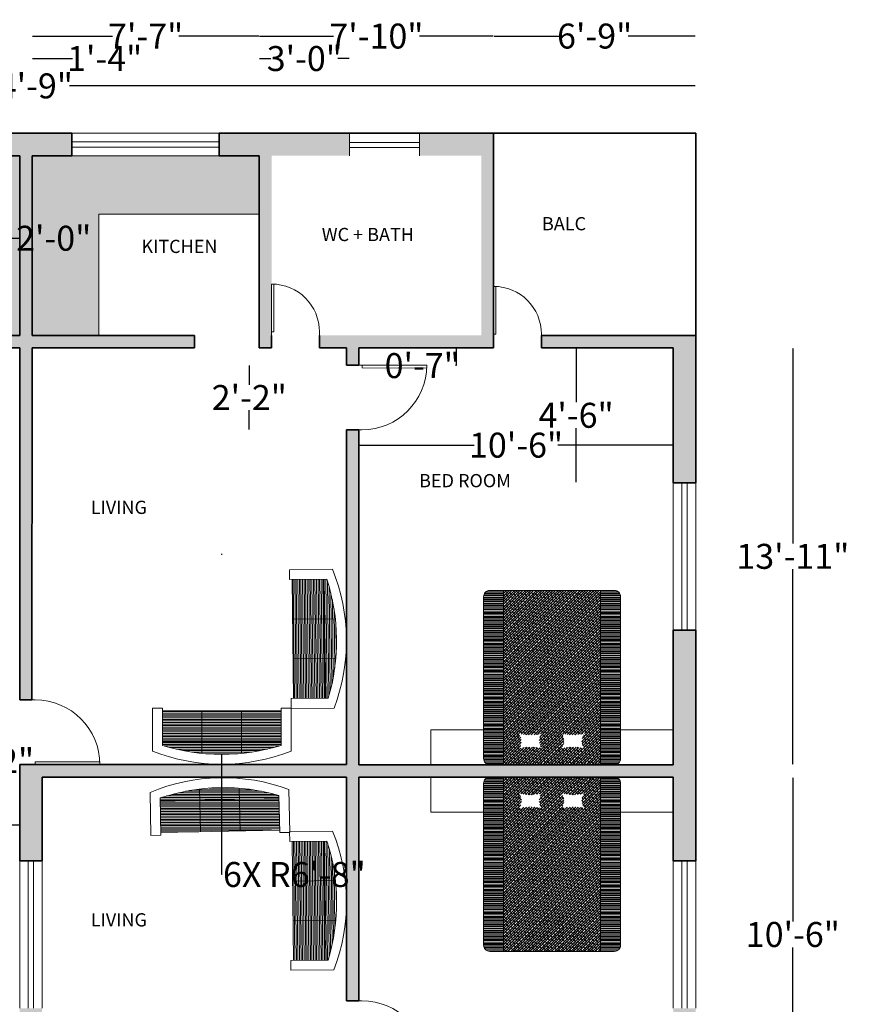
# Model space of a CAD drawing. Units: inches. Extents: x 1198 to 8596, y 144 to 930.
# Tile 5 of 5: x 1614 to 1946, y 536 to 930. Entities that reach past the tile are written whole.
import ezdxf

# ---------------------------------------------------------------- set-up
doc = ezdxf.new("R2010")
doc.units = ezdxf.units.IN
doc.header["$MEASUREMENT"] = 0
doc.layers.get('0').update_dxf_attribs({"color": 50})
for name, color, linetype, lineweight in [('A-ANNO-DIMS', 7, 'Continuous', 18), ('A-AREA-IDEN', 7, 'Continuous', 18), ('A-DOOR', 120, 'Continuous', 18), ('A-FLOR-FIXT', 8, 'Continuous', 18), ('A-FLOR-FIXT-PATT', 150, 'Continuous', 13), ('A-FURN', 11, 'Continuous', 18), ('A-FURN-PATT', 11, 'Continuous', 13), ('A-WALL-PATT', 150, 'Continuous', 13), ('WALL', 7, 'Continuous', 35), ('WINDOW', 2, 'Continuous', 18)]:
    doc.layers.add(name, color=color, linetype=linetype, lineweight=lineweight)
doc.styles.get("Standard").update_dxf_attribs({"font": 'arial.ttf'})
doc.dimstyles.get("Standard").update_dxf_attribs({"dimtxt": 10, "dimasz": 0.18, "dimexe": 0.18, "dimexo": 0.0625, "dimgap": 0.09, "dimtad": 0, "dimtih": 1, "dimtoh": 1, "dimdec": 0, "dimzin": 0, "dimdsep": 46, "dimlunit": 3, "dimtxsty": 'Standard', "dimcen": 0.09, "dimse1": 1, "dimse2": 1, "dimadec": 0, "dimazin": 0, "dimtfac": 1, "dimtdec": 0, "dimtofl": 0, "dimtmove": 0, "dimatfit": 3, "dimfxl": 1, "dimtolj": 1, "dimtzin": 0, "dimarcsym": 0})

# ---------------------------------------------------------------- blocks, each defined once
blk = doc.blocks.new('*D2')
at = {"layer": 'A-ANNO-DIMS', "color": 0, "lineweight": -2, "transparency": 16777216}
for p, q in [((1509.07, 607.65), (1548, 607.65)), ((1613.71, 607.65), (1574.77, 607.65))]:
    blk.add_line(p, q, dxfattribs=at)
at = {"layer": 'A-ANNO-DIMS', "color": 0, "transparency": 16777216}
for points in [[(1509.07, 607.68), (1509.07, 607.62), (1508.89, 607.65)], [(1613.71, 607.68), (1613.71, 607.62), (1613.89, 607.65)]]:
    blk.add_solid(points, dxfattribs=at)
at = {"layer": 'Defpoints', "color": 0, "transparency": 16777216}
for p in [(1508.89, 607.65), (1613.89, 607.65), (1613.89, 607.65)]:
    blk.add_point(p, dxfattribs=at)
at = {"layer": 'A-ANNO-DIMS', "color": 0, "transparency": 16777216, "insert": (1561.39, 607.65), "char_height": 10, "attachment_point": 5}
blk.add_mtext('\\A1;8\'-9"', dxfattribs=at)
blk = doc.blocks.new('WD_WIN4')
for p, q in [((-0.5, 0.5), (0.5, 0.5)), ((-0.5, 0.12), (0.5, 0.12)), ((-0.5, -0.12), (0.5, -0.12)), ((-0.5, -0.5), (0.5, -0.5))]:
    blk.add_line(p, q)
blk = doc.blocks.new('*U10')
for p, q in [((0, 0), (0, -6)), ((-40, 0), (-40, -6))]:
    blk.add_line(p, q)
blk.add_lwpolyline([(0, 0), (0, 40), (-1.75, 40), (-1.75, 0)], close=True)
blk.add_arc((0, 0), 40, 90, 180)
blk = doc.blocks.new('*U11')
for p, q in [((0, 0), (0, -6)), ((40, 0), (40, -6))]:
    blk.add_line(p, q)
blk.add_lwpolyline([(0, 0), (0, 40), (1.75, 40), (1.75, 0)], close=True)
blk.add_arc((0, 0), 40, 0, 90)
blk = doc.blocks.new('*U12')
for p, q in [((0, 0), (0, -6)), ((-40, 0), (-40, -6))]:
    blk.add_line(p, q)
blk.add_lwpolyline([(0, 0), (0, 40), (-1.75, 40), (-1.75, 0)], close=True)
blk.add_arc((0, 0), 40, 90, 180)
blk = doc.blocks.new('Sofa - Roundback 7 ft.')
for p, q in [((-36.000027, -34), (-36.000027, -11.4696)), ((-12.00002, -32.4421), (-12.00003, -6.5971)), ((11.99997, -32.4421), (11.99998, -6.5971)), ((35.99998, -34), (35.99998, -11.4696)), ((-35.999844, -13.3819), (35.9998, -13.3819)), ((-36.000027, -32.4421), (35.99998, -32.4421))]:
    blk.add_line(p, q)
for points in [[(-36.000027, -34), (-42.000027, -34), (-42.000027, -8)], [(41.99998, -8), (41.99998, -34), (35.99998, -34)]]:
    blk.add_lwpolyline(points)
for centre, radius, start, end in [((0, -114.25), 114.25, 68.43141, 111.5686), ((-0.00001, -127.1968), 121.1968, 72.72033, 107.2797)]:
    blk.add_arc(centre, radius, start, end)
blk = doc.blocks.new('*D15')
at = {"layer": 'A-ANNO-DIMS', "color": 0, "lineweight": -2, "transparency": 16777216}
for p, q in [((1348.07, 903.88), (1598.92, 903.88)), ((1884.71, 903.88), (1633.85, 903.88))]:
    blk.add_line(p, q, dxfattribs=at)
at = {"layer": 'A-ANNO-DIMS', "color": 0, "transparency": 16777216}
for points in [[(1348.07, 903.91), (1348.07, 903.85), (1347.89, 903.88)], [(1884.71, 903.91), (1884.71, 903.85), (1884.89, 903.88)]]:
    blk.add_solid(points, dxfattribs=at)
at = {"layer": 'Defpoints', "color": 0, "transparency": 16777216}
for p in [(1347.89, 903.88), (1347.89, 884.9), (1884.89, 884.9)]:
    blk.add_point(p, dxfattribs=at)
at = {"layer": 'A-ANNO-DIMS', "color": 0, "transparency": 16777216, "insert": (1616.39, 903.88), "char_height": 10, "attachment_point": 5}
blk.add_mtext('\\A1;44\'-9"', dxfattribs=at)
blk = doc.blocks.new('WIN-NARROW-28IN')
for p, q in [((0, 9), (0, 0)), ((28.06, 9), (28.06, 0)), ((0, 5.31), (28.06, 5.31)), ((0, 3.31), (28.06, 3.31))]:
    blk.add_line(p, q)
blk = doc.blocks.new('NIGHTSTAND')
for p, q in [((23.07, 13.96), (0, 13.96)), ((23.07, 0), (23.07, 13.96)), ((1.94, 0), (23.07, 0))]:
    blk.add_line(p, q)
blk = doc.blocks.new('*D33')
at = {"layer": 'A-ANNO-DIMS', "color": 0, "lineweight": -2, "transparency": 16777216}
for p, q in [((1619.07, 923.85), (1651.05, 923.85)), ((1709.71, 923.85), (1677.73, 923.85))]:
    blk.add_line(p, q, dxfattribs=at)
at = {"layer": 'A-ANNO-DIMS', "color": 0, "transparency": 16777216}
for points in [[(1619.07, 923.88), (1619.07, 923.82), (1618.89, 923.85)], [(1709.71, 923.88), (1709.71, 923.82), (1709.89, 923.85)]]:
    blk.add_solid(points, dxfattribs=at)
at = {"layer": 'Defpoints', "color": 0, "transparency": 16777216}
for p in [(1709.89, 923.85), (1618.89, 875.9), (1709.89, 875.9)]:
    blk.add_point(p, dxfattribs=at)
at = {"layer": 'A-ANNO-DIMS', "color": 0, "transparency": 16777216, "insert": (1664.39, 923.85), "char_height": 10, "attachment_point": 5}
blk.add_mtext('\\A1;7\'-7"', dxfattribs=at)
blk = doc.blocks.new('*D34')
at = {"layer": 'A-ANNO-DIMS', "color": 0, "lineweight": -2, "transparency": 16777216}
for p, q in [((1710.07, 923.85), (1739.66, 923.85)), ((1803.71, 923.85), (1774.11, 923.85))]:
    blk.add_line(p, q, dxfattribs=at)
at = {"layer": 'A-ANNO-DIMS', "color": 0, "transparency": 16777216}
for points in [[(1710.07, 923.88), (1710.07, 923.82), (1709.89, 923.85)], [(1803.71, 923.88), (1803.71, 923.82), (1803.89, 923.85)]]:
    blk.add_solid(points, dxfattribs=at)
at = {"layer": 'Defpoints', "color": 0, "transparency": 16777216}
for p in [(1803.89, 923.85), (1803.89, 884.9), (1709.89, 875.9)]:
    blk.add_point(p, dxfattribs=at)
at = {"layer": 'A-ANNO-DIMS', "color": 0, "transparency": 16777216, "insert": (1756.89, 923.85), "char_height": 10, "attachment_point": 5}
blk.add_mtext('\\A1;7\'-10"', dxfattribs=at)
blk = doc.blocks.new('*D35')
at = {"layer": 'A-ANNO-DIMS', "color": 0, "lineweight": -2, "transparency": 16777216}
for p, q in [((1804.07, 923.85), (1830.98, 923.85)), ((1884.71, 923.85), (1857.79, 923.85))]:
    blk.add_line(p, q, dxfattribs=at)
at = {"layer": 'A-ANNO-DIMS', "color": 0, "transparency": 16777216}
for points in [[(1804.07, 923.88), (1804.07, 923.82), (1803.89, 923.85)], [(1884.71, 923.88), (1884.71, 923.82), (1884.89, 923.85)]]:
    blk.add_solid(points, dxfattribs=at)
at = {"layer": 'Defpoints', "color": 0, "transparency": 16777216}
for p in [(1884.89, 923.85), (1803.89, 884.9), (1884.89, 884.9)]:
    blk.add_point(p, dxfattribs=at)
at = {"layer": 'A-ANNO-DIMS', "color": 0, "transparency": 16777216, "insert": (1844.39, 923.85), "char_height": 10, "attachment_point": 5}
blk.add_mtext('\\A1;6\'-9"', dxfattribs=at)
blk = doc.blocks.new('*D42')
at = {"layer": 'A-ANNO-DIMS', "color": 0, "lineweight": -2, "transparency": 16777216}
for p, q in [((1750.07, 759.95), (1796.09, 759.95)), ((1875.71, 759.95), (1829.68, 759.95))]:
    blk.add_line(p, q, dxfattribs=at)
at = {"layer": 'A-ANNO-DIMS', "color": 0, "transparency": 16777216}
for points in [[(1750.07, 759.98), (1750.07, 759.92), (1749.89, 759.95)], [(1875.71, 759.98), (1875.71, 759.92), (1875.89, 759.95)]]:
    blk.add_solid(points, dxfattribs=at)
at = {"layer": 'Defpoints', "color": 0, "transparency": 16777216}
for p in [(1749.89, 798.9), (1875.89, 798.9), (1749.89, 759.95)]:
    blk.add_point(p, dxfattribs=at)
at = {"layer": 'A-ANNO-DIMS', "color": 0, "transparency": 16777216, "insert": (1812.89, 759.95), "char_height": 10, "attachment_point": 5}
blk.add_mtext('\\A1;10\'-6"', dxfattribs=at)
blk = doc.blocks.new('*D43')
at = {"layer": 'A-ANNO-DIMS', "color": 0, "lineweight": -2, "transparency": 16777216}
for p, q in [((1923.84, 798.72), (1923.84, 720.6)), ((1923.84, 632.08), (1923.84, 710.2))]:
    blk.add_line(p, q, dxfattribs=at)
at = {"layer": 'A-ANNO-DIMS', "color": 0, "transparency": 16777216}
for points in [[(1923.81, 798.72), (1923.87, 798.72), (1923.84, 798.9)], [(1923.81, 632.08), (1923.87, 632.08), (1923.84, 631.9)]]:
    blk.add_solid(points, dxfattribs=at)
at = {"layer": 'Defpoints', "color": 0, "transparency": 16777216}
for p in [(1875.89, 798.9), (1923.84, 798.9), (1875.89, 631.9)]:
    blk.add_point(p, dxfattribs=at)
at = {"layer": 'A-ANNO-DIMS', "color": 0, "transparency": 16777216, "insert": (1923.84, 715.4), "char_height": 10, "attachment_point": 5}
blk.add_mtext('\\A1;13\'-11"', dxfattribs=at)
blk = doc.blocks.new('*D44')
at = {"layer": 'A-ANNO-DIMS', "color": 0, "lineweight": -2, "transparency": 16777216}
for p, q in [((1923.84, 626.72), (1923.84, 569.09)), ((1923.84, 501.08), (1923.84, 558.7))]:
    blk.add_line(p, q, dxfattribs=at)
at = {"layer": 'A-ANNO-DIMS', "color": 0, "transparency": 16777216}
for points in [[(1923.81, 626.72), (1923.87, 626.72), (1923.84, 626.9)], [(1923.81, 501.08), (1923.87, 501.08), (1923.84, 500.9)]]:
    blk.add_solid(points, dxfattribs=at)
at = {"layer": 'Defpoints', "color": 0, "transparency": 16777216}
for p in [(1875.89, 626.9), (1923.84, 626.9), (1875.89, 500.9)]:
    blk.add_point(p, dxfattribs=at)
at = {"layer": 'A-ANNO-DIMS', "color": 0, "transparency": 16777216, "insert": (1923.84, 563.9), "char_height": 10, "attachment_point": 5}
blk.add_mtext('\\A1;10\'-6"', dxfattribs=at)
blk = doc.blocks.new('*D53')
at = {"layer": 'A-ANNO-DIMS', "color": 0, "lineweight": -2, "transparency": 16777216}
for p, q in [((1800.03, 167.95), (1813.72, 167.95)), ((1854.57, 167.95), (1840.88, 167.95))]:
    blk.add_line(p, q, dxfattribs=at)
at = {"layer": 'A-ANNO-DIMS', "color": 0, "transparency": 16777216}
for points in [[(1800.03, 167.98), (1800.03, 167.92), (1799.85, 167.95)], [(1854.57, 167.98), (1854.57, 167.92), (1854.75, 167.95)]]:
    blk.add_solid(points, dxfattribs=at)
at = {"layer": 'Defpoints', "color": 0, "transparency": 16777216}
for p in [(1799.85, 559.62), (1854.75, 559.62), (1854.75, 167.95)]:
    blk.add_point(p, dxfattribs=at)
at = {"layer": 'A-ANNO-DIMS', "color": 0, "transparency": 16777216, "insert": (1827.3, 167.95), "char_height": 10, "attachment_point": 5}
blk.add_mtext('\\A1;4\'-7"', dxfattribs=at)
blk = doc.blocks.new('*D54')
at = {"layer": 'A-ANNO-DIMS', "color": 0, "lineweight": -2, "transparency": 16777216}
for p, q in [((1308.94, 626.78), (1308.94, 597.25)), ((1308.94, 557.33), (1308.94, 586.85))]:
    blk.add_line(p, q, dxfattribs=at)
at = {"layer": 'A-ANNO-DIMS', "color": 0, "transparency": 16777216}
for points in [[(1308.91, 626.78), (1308.97, 626.78), (1308.94, 626.96)], [(1308.91, 557.33), (1308.97, 557.33), (1308.94, 557.15)]]:
    blk.add_solid(points, dxfattribs=at)
at = {"layer": 'Defpoints', "color": 0, "transparency": 16777216}
for p in [(1308.94, 626.96), (1802.33, 626.96), (1802.33, 557.15)]:
    blk.add_point(p, dxfattribs=at)
at = {"layer": 'A-ANNO-DIMS', "color": 0, "transparency": 16777216, "insert": (1308.94, 592.05), "char_height": 10, "attachment_point": 5}
blk.add_mtext('\\A1;5\'-10"', dxfattribs=at)
blk = doc.blocks.new('*D55')
at = {"layer": 'A-ANNO-DIMS', "color": 0, "lineweight": -2, "transparency": 16777216}
for p, q in [((1710.07, 914.85), (1714.61, 914.85)), ((1745.91, 914.85), (1741.37, 914.85))]:
    blk.add_line(p, q, dxfattribs=at)
at = {"layer": 'A-ANNO-DIMS', "color": 0, "transparency": 16777216}
for points in [[(1710.07, 914.88), (1710.07, 914.82), (1709.89, 914.85)], [(1745.91, 914.88), (1745.91, 914.82), (1746.09, 914.85)]]:
    blk.add_solid(points, dxfattribs=at)
at = {"layer": 'Defpoints', "color": 0, "transparency": 16777216}
for p in [(1746.09, 914.85), (1709.89, 875.9), (1746.09, 875.9)]:
    blk.add_point(p, dxfattribs=at)
at = {"layer": 'A-ANNO-DIMS', "color": 0, "transparency": 16777216, "insert": (1727.99, 914.85), "char_height": 10, "attachment_point": 5}
blk.add_mtext('\\A1;3\'-0"', dxfattribs=at)
blk = doc.blocks.new('*D56')
at = {"layer": 'A-ANNO-DIMS', "color": 0, "lineweight": -2, "transparency": 16777216}
for p, q in [((1619.07, 914.85), (1634.68, 914.85)), ((1634.86, 914.85), (1635.04, 914.85))]:
    blk.add_line(p, q, dxfattribs=at)
at = {"layer": 'A-ANNO-DIMS', "color": 0, "transparency": 16777216}
for points in [[(1619.07, 914.88), (1619.07, 914.82), (1618.89, 914.85)], [(1634.68, 914.88), (1634.68, 914.82), (1634.86, 914.85)]]:
    blk.add_solid(points, dxfattribs=at)
at = {"layer": 'Defpoints', "color": 0, "transparency": 16777216}
for p in [(1634.86, 914.85), (1618.89, 875.9), (1634.86, 875.9)]:
    blk.add_point(p, dxfattribs=at)
at = {"layer": 'A-ANNO-DIMS', "color": 0, "transparency": 16777216, "insert": (1647.95, 914.85), "char_height": 10, "attachment_point": 5}
blk.add_mtext('\\A1;1\'-4"', dxfattribs=at)
blk = doc.blocks.new('*D57')
at = {"layer": 'A-ANNO-DIMS', "color": 0, "lineweight": -2, "transparency": 16777216}
for p, q in [((1836.94, 798.72), (1836.94, 777.11)), ((1836.94, 745.1), (1836.94, 766.71))]:
    blk.add_line(p, q, dxfattribs=at)
at = {"layer": 'A-ANNO-DIMS', "color": 0, "transparency": 16777216}
for points in [[(1836.91, 798.72), (1836.97, 798.72), (1836.94, 798.9)], [(1836.91, 745.1), (1836.97, 745.1), (1836.94, 744.92)]]:
    blk.add_solid(points, dxfattribs=at)
at = {"layer": 'Defpoints', "color": 0, "transparency": 16777216}
for p in [(1836.94, 798.9), (1875.89, 798.9), (1875.89, 744.92)]:
    blk.add_point(p, dxfattribs=at)
at = {"layer": 'A-ANNO-DIMS', "color": 0, "transparency": 16777216, "insert": (1836.94, 771.91), "char_height": 10, "attachment_point": 5}
blk.add_mtext('\\A1;4\'-6"', dxfattribs=at)
blk = doc.blocks.new('*D58')
at = {"layer": 'A-ANNO-DIMS', "color": 0, "lineweight": -2, "transparency": 16777216}
for p, q in [((1788.84, 798.72), (1788.84, 792.18)), ((1788.84, 791.82), (1788.66, 791.82)), ((1788.84, 792), (1788.84, 791.82))]:
    blk.add_line(p, q, dxfattribs=at)
at = {"layer": 'A-ANNO-DIMS', "color": 0, "transparency": 16777216}
for points in [[(1788.81, 798.72), (1788.87, 798.72), (1788.84, 798.9)], [(1788.81, 792.18), (1788.87, 792.18), (1788.84, 792)]]:
    blk.add_solid(points, dxfattribs=at)
at = {"layer": 'Defpoints', "color": 0, "transparency": 16777216}
for p in [(1749.89, 798.9), (1749.89, 792), (1788.84, 792)]:
    blk.add_point(p, dxfattribs=at)
at = {"layer": 'A-ANNO-DIMS', "color": 0, "transparency": 16777216, "insert": (1775.27, 791.82), "char_height": 10, "attachment_point": 5}
blk.add_mtext('\\A1;0\'-7"', dxfattribs=at)
blk = doc.blocks.new('*D59')
at = {"layer": 'A-ANNO-DIMS', "color": 0, "lineweight": -2, "transparency": 16777216}
for p, q in [((1705.94, 791.82), (1705.94, 784.15)), ((1705.94, 766.26), (1705.94, 773.93))]:
    blk.add_line(p, q, dxfattribs=at)
at = {"layer": 'A-ANNO-DIMS', "color": 0, "transparency": 16777216}
for points in [[(1705.91, 791.82), (1705.97, 791.82), (1705.94, 792)], [(1705.91, 766.26), (1705.97, 766.26), (1705.94, 766.08)]]:
    blk.add_solid(points, dxfattribs=at)
at = {"layer": 'Defpoints', "color": 0, "transparency": 16777216}
for p in [(1705.94, 792), (1744.89, 792), (1744.89, 766.08)]:
    blk.add_point(p, dxfattribs=at)
at = {"layer": 'A-ANNO-DIMS', "color": 0, "transparency": 16777216, "insert": (1705.94, 779.04), "char_height": 10, "attachment_point": 5}
blk.add_mtext('\\A1;2\'-2"', dxfattribs=at)
blk = doc.blocks.new('*D61')
at = {"layer": 'A-ANNO-DIMS', "color": 0, "lineweight": -2, "transparency": 16777216}
for p, q in [((1589.91, 842.85), (1613.71, 842.85)), ((1613.89, 842.85), (1614.07, 842.85))]:
    blk.add_line(p, q, dxfattribs=at)
at = {"layer": 'A-ANNO-DIMS', "color": 0, "transparency": 16777216}
for points in [[(1589.91, 842.88), (1589.91, 842.82), (1589.73, 842.85)], [(1613.71, 842.88), (1613.71, 842.82), (1613.89, 842.85)]]:
    blk.add_solid(points, dxfattribs=at)
at = {"layer": 'Defpoints', "color": 0, "transparency": 16777216}
for p in [(1613.89, 842.85), (1589.73, 803.9), (1613.89, 803.9)]:
    blk.add_point(p, dxfattribs=at)
at = {"layer": 'A-ANNO-DIMS', "color": 0, "transparency": 16777216, "insert": (1627.53, 842.85), "char_height": 10, "attachment_point": 5}
blk.add_mtext('\\A1;2\'-0"', dxfattribs=at)
blk = doc.blocks.new('*D69')
at = {"layer": 'A-ANNO-DIMS', "color": 0, "lineweight": -2, "transparency": 16777216}
for p, q in [((1538.43, 754.55), (1538.61, 754.55)), ((1538.52, 754.46), (1538.52, 754.64)), ((1538.53, 633.54), (1538.53, 678.74)), ((1538.71, 633.54), (1538.53, 633.54))]:
    blk.add_line(p, q, dxfattribs=at)
at = {"layer": 'A-ANNO-DIMS', "color": 0, "transparency": 16777216}
blk.add_solid([(1538.56, 678.74), (1538.5, 678.74), (1538.53, 678.92)], dxfattribs=at)
at = {"layer": 'Defpoints', "color": 0, "transparency": 16777216}
for p in [(1538.52, 754.55), (1538.53, 678.92)]:
    blk.add_point(p, dxfattribs=at)
at = {"layer": 'A-ANNO-DIMS', "color": 0, "transparency": 16777216, "insert": (1579.29, 633.54), "char_height": 10, "attachment_point": 5}
blk.add_mtext('\\A1;6X R6\'-3 1/2"', dxfattribs=at)
blk = doc.blocks.new('*D70')
at = {"layer": 'A-ANNO-DIMS', "color": 0, "lineweight": -2, "transparency": 16777216}
for p, q in [((1694.82, 716.29), (1695, 716.29)), ((1694.91, 716.2), (1694.91, 716.38)), ((1694.91, 587.93), (1694.91, 635.88)), ((1695.09, 587.93), (1694.91, 587.93))]:
    blk.add_line(p, q, dxfattribs=at)
at = {"layer": 'A-ANNO-DIMS', "color": 0, "transparency": 16777216}
blk.add_solid([(1694.94, 635.88), (1694.88, 635.88), (1694.91, 636.06)], dxfattribs=at)
at = {"layer": 'Defpoints', "color": 0, "transparency": 16777216}
for p in [(1694.91, 716.29), (1694.91, 636.06)]:
    blk.add_point(p, dxfattribs=at)
at = {"layer": 'A-ANNO-DIMS', "color": 0, "transparency": 16777216, "insert": (1724.02, 587.93), "char_height": 10, "attachment_point": 5}
blk.add_mtext('\\A1;6X R6\'-8"', dxfattribs=at)

msp = doc.modelspace()

# ---------------------------------------------------------------- hatches: boundary and pattern name
at = {"layer": 'A-FLOR-FIXT-PATT', "transparency": 33554607}
h = msp.add_hatch(dxfattribs=at)
h.set_pattern_fill('ACAD_ISO04W100', color=256, scale=0.1)
h.set_pattern_definition([(0, (0, 0), (0, 0.5), [2.4, -0.3, 0.05, -0.3])])
h.paths.add_polyline_path([(1613.89, 875.9), (1597.91, 875.9), (1538.86, 875.9), (1522.89, 875.9), (1522.89, 849.66), (1589.73, 849.66), (1589.73, 803.9), (1613.89, 803.9)])
h.paths.add_polyline_path([(1709.89, 875.9), (1693.91, 875.9), (1634.86, 875.9), (1618.89, 875.9), (1618.89, 803.9), (1645.58, 803.9), (1645.58, 852.52), (1709.89, 852.52)])
at = {"layer": 'A-FURN-PATT'}
h = msp.add_hatch(dxfattribs=at)
h.set_pattern_fill('LINE', color=256, scale=5, angle=90.6803)
h.set_pattern_definition([(90.6803, (2441.98376, -846.3033), (-0.62495594, -0.00742075), [])])
h.paths.add_polyline_path([(1723.51, 674.3), (1723.69, 658.42), (1736.31, 658.56), (1736.12, 674.45)])
h.paths.add_polyline_path([(1723.32, 690.19), (1723.51, 674.3), (1736.12, 674.45), (1735.93, 690.34)])
h.paths.add_polyline_path([(1723.13, 706.07), (1723.32, 690.19), (1735.93, 690.34), (1735.75, 706.22)])
h.paths.add_polyline_path([(1737.01, 706.24), (1735.75, 706.22), (1735.93, 690.34), (1740.43, 690.39, 0.050647)])
h.paths.add_polyline_path([(1735.93, 690.34), (1736.12, 674.45), (1740.61, 674.5, 0.049628), (1740.43, 690.39)])
h.paths.add_polyline_path([(1736.12, 674.45), (1736.31, 658.56), (1737.58, 658.58, 0.050647), (1740.61, 674.5)])
h = msp.add_hatch(dxfattribs=at)
h.set_pattern_fill('PLASTI', color=256, scale=6.190048)
h.set_pattern_definition([(0, (526.78, 220.506), (0, 1.547512), []), (0, (526.78, 220.6994), (0, 1.547512), []), (0, (526.78, 220.8928), (0, 1.547512), []), (0, (526.78, 221.4731), (0, 1.547512), [])])
h.paths.add_polyline_path([(1846.77, 631.9), (1852.27, 631.9, 0.414214), (1854.75, 634.37), (1854.75, 699.23, 0.414214), (1852.27, 701.71), (1846.77, 701.71)])
h.paths.add_polyline_path([(1799.85, 634.37, 0.414214), (1802.33, 631.9), (1807.83, 631.9), (1807.83, 701.71), (1802.33, 701.71, 0.414214), (1799.85, 699.23)])
h = msp.add_hatch(dxfattribs=at)
h.set_pattern_fill('ANSI38', color=256, scale=6.190048)
h.set_pattern_definition([(45, (526.78, 220.5059), (-0.5471281, 0.5471281), []), (135, (526.78, 220.5059), (-1.6413843, 0.5471281), [1.93439, -1.160634])])
h.paths.add_polyline_path([(1807.83, 631.9), (1846.77, 631.9), (1846.77, 701.71), (1807.83, 701.71)])
h.paths.add_polyline_path([(1823.26, 644.41, 0.358285), (1823.26, 638.41, 0.116256), (1813.93, 638.41, 0.358285), (1813.93, 644.41, 0.116256)], flags=16)
h.paths.add_polyline_path([(1831.01, 644.41, 0.116256), (1840.34, 644.41, 0.358285), (1840.34, 638.41, 0.116256), (1831.01, 638.41, 0.358285)], flags=16)
h = msp.add_hatch(dxfattribs=at)
h.set_pattern_fill('LINE', color=256, scale=5)
h.set_pattern_definition([(0, (157.9337, -46.80456), (0, 0.625), [])])
h.paths.add_polyline_path([(1686.96, 653.57), (1671.07, 653.57), (1671.07, 640.95), (1686.96, 640.95)])
h.paths.add_polyline_path([(1702.85, 653.57), (1686.96, 653.57), (1686.96, 640.95), (1702.85, 640.95)])
h.paths.add_polyline_path([(1718.74, 653.57), (1702.85, 653.57), (1702.85, 640.95), (1718.74, 640.95)])
h.paths.add_polyline_path([(1718.74, 639.68), (1718.74, 640.95), (1702.85, 640.95), (1702.85, 636.46, 0.050647)])
h.paths.add_polyline_path([(1702.85, 640.95), (1686.96, 640.95), (1686.96, 636.46, 0.049628), (1702.85, 636.46)])
h.paths.add_polyline_path([(1686.96, 640.95), (1671.07, 640.95), (1671.07, 639.68, 0.050647), (1686.96, 636.46)])
h = msp.add_hatch(dxfattribs=at)
h.set_pattern_fill('PLASTI', color=256, scale=6.190048)
h.set_pattern_definition([(0, (526.78, 224.1068), (0, 1.547512), []), (0, (526.78, 224.3002), (0, 1.547512), []), (0, (526.78, 224.4937), (0, 1.547512), []), (0, (526.78, 225.074), (0, 1.547512), [])])
h.paths.add_polyline_path([(1846.77, 557.15), (1852.27, 557.15, 0.414214), (1854.75, 559.62), (1854.75, 624.48, 0.414214), (1852.27, 626.96), (1846.77, 626.96)])
h.paths.add_polyline_path([(1799.85, 559.62, 0.414214), (1802.33, 557.15), (1807.83, 557.15), (1807.83, 626.96), (1802.33, 626.96, 0.414214), (1799.85, 624.48)])
h = msp.add_hatch(dxfattribs=at)
h.set_pattern_fill('ANSI38', color=256, scale=6.190048)
h.set_pattern_definition([(45, (526.78, 224.1068), (-0.5471281, 0.5471281), []), (135, (526.78, 224.1068), (-1.6413843, 0.5471281), [1.93439, -1.160634])])
h.paths.add_polyline_path([(1807.83, 557.15), (1846.77, 557.15), (1846.77, 626.96), (1807.83, 626.96)])
h.paths.add_polyline_path([(1823.26, 614.44, 0.116256), (1813.93, 614.44, 0.358285), (1813.93, 620.44, 0.116256), (1823.26, 620.44, 0.358285)], flags=16)
h.paths.add_polyline_path([(1831.01, 614.44, 0.358285), (1831.01, 620.44, 0.116256), (1840.34, 620.44, 0.358285), (1840.34, 614.44, 0.116256)], flags=16)
h = msp.add_hatch(dxfattribs=at)
h.set_pattern_fill('LINE', color=256, scale=5)
h.set_pattern_definition([(0, (156.7616, -42.46536), (0, 0.625), [])])
h.paths.add_polyline_path([(1686.36, 605.05), (1670.47, 604.71), (1670.2, 617.32), (1686.09, 617.66)])
h.paths.add_polyline_path([(1702.24, 605.39), (1686.36, 605.05), (1686.09, 617.66), (1701.97, 618.01)])
h.paths.add_polyline_path([(1718.13, 605.73), (1702.24, 605.39), (1701.97, 618.01), (1717.85, 618.35)])
h.paths.add_polyline_path([(1717.83, 619.61), (1717.85, 618.35), (1701.97, 618.01), (1701.87, 622.5, -0.050647)])
h.paths.add_polyline_path([(1701.97, 618.01), (1686.09, 617.66), (1685.99, 622.16, -0.049628), (1701.87, 622.5)])
h.paths.add_polyline_path([(1686.09, 617.66), (1670.2, 617.32), (1670.18, 618.59, -0.050647), (1685.99, 622.16)])
h = msp.add_hatch(dxfattribs=at)
h.set_pattern_fill('LINE', color=256, scale=5, angle=90.6803)
h.set_pattern_definition([(90.6803, (2440.8076, -841.7595), (-0.62495594, -0.00742075), [])])
h.paths.add_polyline_path([(1723.33, 585.31), (1723.18, 601.2), (1735.8, 601.32), (1735.95, 585.43)])
h.paths.add_polyline_path([(1723.49, 569.42), (1723.33, 585.31), (1735.95, 585.43), (1736.1, 569.55)])
h.paths.add_polyline_path([(1723.64, 553.54), (1723.49, 569.42), (1736.1, 569.55), (1736.26, 553.66)])
h.paths.add_polyline_path([(1737.52, 553.67), (1736.26, 553.66), (1736.1, 569.55), (1740.6, 569.59, -0.050647)])
h.paths.add_polyline_path([(1736.1, 569.55), (1735.95, 585.43), (1740.44, 585.48, -0.049628), (1740.6, 569.59)])
h.paths.add_polyline_path([(1735.95, 585.43), (1735.8, 601.32), (1737.06, 601.33, -0.050647), (1740.44, 585.48)])
at = {"layer": 'A-WALL-PATT'}
h = msp.add_hatch(color=256, dxfattribs=at)
h.dxf.hatch_style = 1
h.paths.add_polyline_path([(1884.89, 495.9), (1884.89, 534.37), (1875.89, 534.37), (1875.89, 500.9), (1823.11, 500.9), (1823.11, 495.9)])
h.paths.add_polyline_path([(1875.89, 593.42), (1884.89, 593.42), (1884.89, 685.87), (1875.89, 685.87), (1875.89, 631.9), (1749.89, 631.9), (1749.89, 766.08), (1744.89, 766.08), (1744.89, 631.97), (1618.79, 631.97), (1613.89, 631.97), (1613.89, 593.42), (1622.89, 593.42), (1622.89, 626.9), (1744.89, 626.9), (1744.89, 537.33), (1749.89, 537.33), (1749.89, 626.9), (1875.89, 626.9)])
h.paths.add_polyline_path([(1884.89, 206.9), (1884.89, 249.37), (1875.89, 249.37), (1875.89, 215.9), (1842.41, 215.9), (1842.41, 206.9)])
h.paths.add_polyline_path([(1783.36, 206.9), (1783.36, 215.9), (1749.89, 215.9), (1749.89, 308.42), (1744.89, 308.42), (1744.89, 215.9), (1713.41, 215.9), (1713.41, 206.9)])
h.paths.add_polyline_path([(1654.36, 206.9), (1654.36, 215.9), (1622.89, 215.9), (1622.89, 249.37), (1613.89, 249.37), (1613.89, 206.9)])
h.paths.add_polyline_path([(1613.89, 334.34), (1622.89, 334.34), (1622.89, 341.9), (1622.89, 368.41), (1613.89, 368.41)])
h.paths.add_polyline_path([(1613.89, 396.47), (1622.89, 396.47), (1622.89, 418.9), (1710.09, 418.9), (1710.09, 400.51), (1709.89, 346.77), (1709.89, 341.9), (1714.89, 341.9), (1714.89, 346.9), (1714.88, 366), (1714.89, 418.9), (1798.89, 418.9), (1798.89, 346.9), (1734.06, 346.9), (1734.07, 343.96), (1734.06, 341.9), (1744.89, 341.9), (1744.89, 334.34), (1749.89, 334.34), (1749.89, 341.9), (1803.93, 341.9), (1803.93, 346.9), (1803.89, 346.9), (1803.89, 418.9), (1884.89, 418.9), (1884.89, 423.9), (1803.89, 423.9), (1803.89, 495.9), (1803.93, 500.9), (1749.89, 500.9), (1749.89, 511.41), (1747.24, 511.41), (1744.89, 511.41), (1744.89, 500.9), (1734.06, 500.9), (1734.06, 495.9), (1798.89, 495.9), (1798.89, 423.9), (1714.89, 423.9), (1714.89, 495.9), (1714.89, 500.9), (1709.89, 500.9), (1709.89, 496.89), (1709.89, 495.9), (1709.89, 423.9), (1622.89, 423.9), (1622.89, 446.07), (1613.89, 446.07)])
h.paths.add_polyline_path([(1613.89, 474.13), (1622.89, 474.13), (1622.89, 495.9), (1645.93, 495.9), (1683.97, 495.9), (1683.89, 500.9), (1648.32, 500.9), (1648.32, 500.88), (1622.41, 500.86), (1618.52, 500.86), (1613.89, 500.9)])
h.paths.add_polyline_path([(1613.89, 526.77), (1613.89, 534.37), (1622.89, 534.37), (1622.89, 526.77, -0.395914), (1648.3, 502.01), (1648.32, 502.01), (1648.32, 500.88), (1622.41, 500.86), (1622.41, 502), (1648.3, 502.01, 0.395914), (1622.89, 526.77)])
h.paths.add_polyline_path([(1875.89, 744.92), (1884.89, 744.92), (1884.89, 803.9), (1823.06, 803.9), (1823.06, 798.9), (1875.89, 798.9)])
h.paths.add_polyline_path([(1798.89, 803.9), (1734.06, 803.9), (1734.06, 802.45), (1734.06, 798.9), (1744.89, 798.9), (1744.89, 792), (1749.89, 792), (1749.89, 798.9), (1803.89, 798.9), (1803.89, 803.9), (1803.89, 884.9), (1774.16, 884.9), (1774.16, 875.9), (1798.89, 875.9)])
h.paths.add_polyline_path([(1746.09, 875.9), (1746.09, 884.9), (1693.91, 884.9), (1693.91, 875.9), (1709.89, 875.9), (1709.89, 803.9), (1709.89, 798.9), (1714.89, 798.9), (1714.89, 803.9), (1714.89, 875.9)])
h.paths.add_polyline_path([(1618.89, 798.9), (1683.96, 798.9), (1683.96, 803.9), (1618.89, 803.9), (1618.89, 875.9), (1634.86, 875.9), (1634.86, 884.9), (1597.91, 884.9), (1597.91, 875.9), (1613.89, 875.9), (1613.89, 803.9), (1548.75, 803.9), (1548.75, 798.9), (1613.89, 798.9), (1613.89, 657.88), (1618.8, 657.88)])
h.paths.add_polyline_path([(1522.89, 875.9), (1538.86, 875.9), (1538.86, 884.9), (1483.76, 884.9), (1483.76, 875.9), (1517.89, 875.9), (1517.89, 803.9), (1517.89, 802.46), (1517.89, 798.9), (1522.89, 798.9), (1522.89, 803.9)], flags=17)
h.paths.add_polyline_path([(1428.89, 884.9), (1428.89, 803.9), (1428.89, 798.9), (1482.89, 798.9), (1482.89, 678.9), (1356.89, 678.9), (1356.89, 709.37), (1347.89, 709.37), (1347.89, 577.9), (1508.89, 577.9), (1508.89, 586.9), (1356.89, 586.9), (1356.89, 673.9), (1565.89, 673.9), (1565.89, 678.9), (1487.89, 678.9), (1487.89, 798.9), (1498.72, 798.9), (1498.72, 803.9), (1433.89, 803.9), (1433.89, 875.9), (1455.69, 875.9), (1455.69, 884.9)])
h.paths.add_polyline_path([(1356.89, 798.9), (1409.72, 798.9), (1409.72, 803.9), (1347.89, 803.9), (1347.89, 768.42), (1356.89, 768.42)], flags=17)
h.paths.add_polyline_path([(1884.89, 346.9), (1823.09, 346.9, -0.008805), (1823.1, 346.22), (1823.11, 343.35), (1823.09, 341.9), (1875.89, 341.9), (1875.89, 308.42), (1884.89, 308.42)])

# ---------------------------------------------------------------- linework, layer by layer
at = {"layer": 'A-FLOR-FIXT'}
for p, q in [((1645.58, 803.9), (1645.58, 852.52)), ((1645.58, 852.52), (1709.89, 852.52))]:
    msp.add_line(p, q, dxfattribs=at)
at = {"layer": 'A-FURN'}
for p, q in [((1807.83, 631.9), (1807.83, 701.71)), ((1846.77, 631.9), (1846.77, 701.71)), ((1807.83, 626.96), (1807.83, 557.15)), ((1846.77, 626.96), (1846.77, 557.15))]:
    msp.add_line(p, q, dxfattribs=at)
for points in [[(1802.33, 631.9), (1852.27, 631.9, 0.414214), (1854.75, 634.37), (1854.75, 699.23, 0.414214), (1852.27, 701.71), (1802.33, 701.71, 0.414214), (1799.85, 699.23), (1799.85, 634.37, 0.414214)], [(1802.33, 626.96), (1852.27, 626.96, -0.414214), (1854.75, 624.48), (1854.75, 559.62, -0.414214), (1852.27, 557.15), (1802.33, 557.15, -0.414214), (1799.85, 559.62), (1799.85, 624.48, -0.414214)]]:
    msp.add_lwpolyline(points, format="xyb", close=True, dxfattribs=at)
at = {"layer": 'WALL'}
for p, q in [((1597.91, 884.9), (1634.86, 884.9)), ((1634.86, 875.9), (1634.86, 884.9)), ((1693.91, 884.9), (1884.89, 884.9)), ((1693.91, 875.9), (1693.91, 884.9)), ((1803.89, 803.9), (1803.89, 884.9)), ((1884.89, 744.92), (1884.89, 884.9)), ((1597.91, 875.9), (1613.89, 875.9)), ((1613.89, 803.9), (1613.89, 875.9)), ((1618.89, 875.9), (1634.86, 875.9)), ((1618.89, 803.9), (1618.89, 875.9)), ((1693.91, 875.9), (1709.89, 875.9)), ((1709.89, 803.9), (1709.89, 875.9)), ((1548.75, 803.9), (1613.89, 803.9)), ((1618.89, 803.9), (1683.96, 803.9)), ((1683.96, 803.9), (1683.96, 798.9)), ((1709.89, 803.9), (1709.89, 798.9)), ((1714.89, 803.9), (1714.89, 798.9)), ((1734.06, 803.89), (1734.06, 798.9)), ((1803.89, 803.9), (1803.89, 798.9)), ((1823.06, 803.9), (1884.89, 803.9)), ((1823.06, 803.9), (1823.06, 798.9)), ((1548.75, 798.9), (1613.89, 798.9)), ((1613.89, 798.9), (1613.89, 657.88)), ((1618.89, 798.9), (1618.8, 657.88)), ((1683.96, 798.9), (1618.89, 798.9)), ((1714.89, 798.9), (1709.89, 798.9)), ((1744.89, 798.9), (1734.06, 798.9)), ((1744.89, 792), (1744.89, 798.9)), ((1749.89, 798.9), (1803.89, 798.9)), ((1749.89, 792), (1749.89, 798.9)), ((1823.06, 798.9), (1875.89, 798.9)), ((1875.89, 744.92), (1875.89, 798.9)), ((1749.89, 792), (1744.89, 792)), ((1744.89, 631.97), (1744.89, 766.08)), ((1749.89, 766.08), (1744.89, 766.08)), ((1749.89, 631.9), (1749.89, 766.08)), ((1875.89, 744.92), (1884.89, 744.92)), ((1875.89, 631.9), (1875.89, 685.87)), ((1875.89, 685.87), (1884.89, 685.87)), ((1884.89, 593.42), (1884.89, 685.87)), ((1618.8, 657.88), (1613.89, 657.88)), ((1618.79, 631.97), (1613.89, 631.97)), ((1613.89, 631.97), (1613.89, 593.42)), ((1618.79, 631.97), (1744.89, 631.97)), ((1749.89, 631.9), (1875.89, 631.9)), ((1622.89, 626.9), (1744.89, 626.9)), ((1622.89, 593.42), (1622.89, 626.9)), ((1744.89, 537.33), (1744.89, 626.9)), ((1749.89, 626.9), (1875.89, 626.9)), ((1749.89, 537.33), (1749.89, 626.9)), ((1875.89, 593.42), (1875.89, 626.9)), ((1622.89, 593.42), (1613.89, 593.42)), ((1875.89, 593.42), (1884.89, 593.42)), ((1749.89, 537.33), (1744.89, 537.33))]:
    msp.add_line(p, q, dxfattribs=at)

# ---------------------------------------------------------------- block references
at = {"layer": 'A-DOOR'}
for name, p, xscale, yscale, zscale, rotation in [('*U12', (1714.89, 805.33), -0.4792807635590344, 0.4792807635590344, 0.4792807635590344, 359.9658956660211), ('*U12', (1803.89, 804.4), -0.4792807635590344, 0.4792807635590344, 0.4792807635590344, 359.9658956660211), ('*U10', (1751.13, 792), -0.6478828703427376, 0.6478828703427376, 0.6478828703427376, 269.9658956660211), ('*U11', (1620.13, 631.97), -0.6478828703427376, 0.6478828703427376, 0.6478828703427376, 269.9658956660211), ('*U10', (1751.13, 511.41), 0.6478828703427376, 0.6478828703427376, 0.6478828703427376, 270.0341043339827)]:
    msp.add_blockref(name, p, dxfattribs=dict(at, xscale=xscale, yscale=yscale, zscale=zscale, rotation=rotation))
at = {"layer": 'A-FURN', "yscale": 0.6619781710857556, "zscale": 0.6619781710857556}
for p, xscale, rotation in [((1744.89, 682.5), 0.6619781710857556, 270.6803002411188), ((1694.91, 632.09), 0.6619781710857556, 179.9999999999996), ((1693.84, 626.69), -0.6619781710857556, 1.231183246104441), ((1744.89, 577.57), -0.6619781710857553, 270.5508830049851)]:
    msp.add_blockref('Sofa - Roundback 7 ft.', p, dxfattribs=dict(at, xscale=xscale, rotation=rotation))
at = {"layer": 'A-FURN', "rotation": 180}
msp.add_blockref('NIGHTSTAND', (1801.79, 645.91), dxfattribs=at)
at = {"layer": 'A-FURN', "extrusion": (0, 0, -1), "zscale": -1, "rotation": 180}
msp.add_blockref('NIGHTSTAND', (-1852.81, 645.91), dxfattribs=at)
at = {"layer": 'A-FURN', "extrusion": (0, 0, -1), "zscale": -1}
msp.add_blockref('NIGHTSTAND', (-1801.79, 612.94), dxfattribs=at)
at = {"layer": 'A-FURN'}
msp.add_blockref('NIGHTSTAND', (1852.81, 612.94), dxfattribs=at)
at = {"layer": 'WINDOW', "xscale": 59.05511811023622, "yscale": 9.00000000000125, "zscale": 59.05511811023622}
msp.add_blockref('WD_WIN4', (1664.39, 880.4), dxfattribs=at)
at = {"layer": 'WINDOW'}
msp.add_blockref('WIN-NARROW-28IN', (1746.09, 875.9), dxfattribs=at)
at = {"layer": 'WINDOW', "xscale": 59.05511811023622, "zscale": 59.05511811023622}
for p, yscale, rotation in [((1880.39, 715.4), 9, 269.9999999999998), ((1618.39, 563.9), 8.999999999999773, 90.00000000000351), ((1880.39, 563.9), 8.999999999988859, 270.0000000000092)]:
    msp.add_blockref('WD_WIN4', p, dxfattribs=dict(at, yscale=yscale, rotation=rotation))

# ---------------------------------------------------------------- texts
at = {"layer": 'A-AREA-IDEN'}
for s, p in [('BALC', (1823.26, 846.03)), ('WC + BATH', (1734.98, 841.7)), (' KITCHEN', (1661.06, 836.93)), (' BED ROOM', (1772.4, 743.08)), (' LIVING', (1640.75, 732.39)), (' LIVING', (1640.75, 567.11))]:
    msp.add_text(s, height=5.299, dxfattribs=at).set_placement(p)

# ---------------------------------------------------------------- dimensions: what is measured, and where the dimension line sits
at = {"layer": 'A-ANNO-DIMS'}
for base, p1, p2, override, picture, middle in [((1709.89, 923.85), (1618.89, 875.9), (1709.89, 875.9), {"dimdec": 1, "dimlfac": 1, "dimrnd": 0, "dimzin": 1, "dimdsep": 46, "dimlunit": 4, "dimfrac": 2}, '*D33', (1664.39, 923.85)), ((1803.89, 923.85), (1709.89, 875.9), (1803.89, 884.9), {"dimdec": 1, "dimlfac": 1, "dimrnd": 0, "dimzin": 1, "dimdsep": 46, "dimlunit": 4, "dimfrac": 2}, '*D34', (1756.89, 923.85)), ((1884.89, 923.85), (1803.89, 884.9), (1884.89, 884.9), {"dimdec": 1, "dimlfac": 1, "dimrnd": 0, "dimzin": 1, "dimdsep": 46, "dimlunit": 4, "dimfrac": 2}, '*D35', (1844.39, 923.85)), ((1634.86, 914.85), (1618.89, 875.9), (1634.86, 875.9), {"dimdec": 1, "dimlfac": 1, "dimrnd": 0, "dimzin": 1, "dimdsep": 46, "dimlunit": 4, "dimfrac": 2}, '*D56', (1647.95, 914.85)), ((1746.09, 914.85), (1709.89, 875.9), (1746.09, 875.9), {"dimdec": 1, "dimlfac": 1, "dimrnd": 0, "dimzin": 1, "dimdsep": 46, "dimlunit": 4, "dimfrac": 2}, '*D55', (1727.99, 914.85)), ((1347.89, 903.88), (1884.89, 884.9), (1347.89, 884.9), {"dimclrd": 0, "dimclre": 0, "dimclrt": 0}, '*D15', (1616.39, 903.88)), ((1613.89, 607.65), (1508.89, 607.65), (1613.89, 607.65), {"dimclrd": 0, "dimclre": 0, "dimclrt": 0}, '*D2', (1561.39, 607.65)), ((1854.75, 167.95), (1799.85, 559.62), (1854.75, 559.62), {"dimdec": 1, "dimlfac": 1, "dimrnd": 0, "dimzin": 1, "dimdsep": 46, "dimlunit": 4, "dimfrac": 2}, '*D53', (1827.3, 167.95))]:
    dim = msp.add_linear_dim(base=base, p1=p1, p2=p2, dimstyle='Standard', override=override, dxfattribs=at)
    dim.commit()
    dim.dimension.update_dxf_attribs({"geometry": picture, "text_midpoint": middle})
for base, p1, p2, angle, picture, middle in [((1613.89, 842.85), (1589.73, 803.9), (1613.89, 803.9), 0, '*D61', (1627.53, 842.85)), ((1749.89, 759.95), (1875.89, 798.9), (1749.89, 798.9), 180, '*D42', (1812.89, 759.95)), ((1788.84, 792), (1749.89, 798.9), (1749.89, 792), 270, '*D58', (1775.27, 791.82)), ((1836.94, 798.9), (1875.89, 744.92), (1875.89, 798.9), 90, '*D57', (1836.94, 771.91)), ((1923.84, 798.9), (1875.89, 631.9), (1875.89, 798.9), 90, '*D43', (1923.84, 715.4)), ((1705.94, 792), (1744.89, 766.08), (1744.89, 792), 90, '*D59', (1705.94, 779.04)), ((1308.94, 626.96), (1802.33, 557.15), (1802.33, 626.96), 90, '*D54', (1308.94, 592.05)), ((1923.84, 626.9), (1875.89, 500.9), (1875.89, 626.9), 90, '*D44', (1923.84, 563.9))]:
    dim = msp.add_linear_dim(base=base, p1=p1, p2=p2, angle=angle, dimstyle='Standard', override={"dimdec": 1, "dimlfac": 1, "dimrnd": 0, "dimzin": 1, "dimdsep": 46, "dimlunit": 4, "dimfrac": 2}, dxfattribs=at)
    dim.commit()
    dim.dimension.update_dxf_attribs({"geometry": picture, "text_midpoint": middle})
for center, mpoint, picture, middle in [((1538.52, 754.55), (1538.53, 678.92), '*D69', (1579.29, 633.54)), ((1694.91, 716.29), (1694.91, 636.06), '*D70', (1724.02, 587.93))]:
    dim = msp.add_radius_dim(center=center, mpoint=mpoint, text='6X <>', dimstyle='Standard', override={"dimdec": 1, "dimlfac": 1, "dimrnd": 0, "dimzin": 1, "dimdsep": 46, "dimlunit": 4, "dimfrac": 2}, dxfattribs=at)
    dim.commit()
    dim.dimension.update_dxf_attribs({"geometry": picture, "text_midpoint": middle, "dimtype": 164})

doc.saveas('drawing.dxf')
